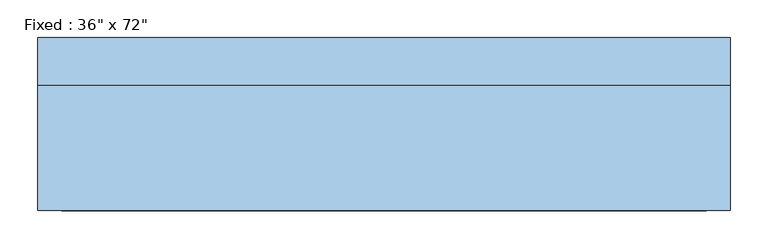
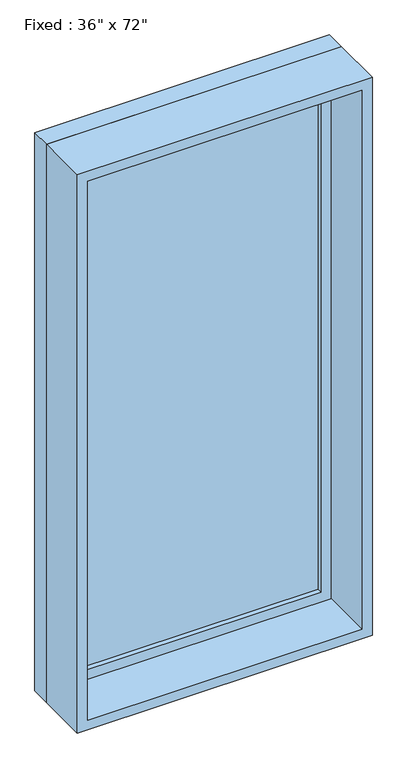
"""IFC4 building model written with IfcOpenShell, lengths in millimetres: window geometry."""

from ifc_helpers import new_model, si_unit, frame, origin, place, context, project, spatial, polyline, outline, extrude, source, transform, mapped, element, save


def window_c796fc87(model_context):
    return source(origin(), model_context, "Body", "SweptSolid", [
        extrude(outline(polyline([(355.6, 66.675), (-431.8, 66.675), (-431.8, 79.375), (355.6, 79.375), (355.6, 66.675)])), frame((0.0, 0.0, 368.3), z_axis=(0.0, 0.0, 1.0), x_axis=(1.0, 0.0, 0.0)), (0.0, 0.0, 1.0), 1701.8),
        extrude(outline(polyline([(2114.55, -476.25), (323.85, -476.25), (323.85, 400.05), (2114.55, 400.05), (2114.55, -476.25)]), holes=[polyline([(2070.1, -431.8), (2070.1, 355.6), (368.3, 355.6), (368.3, -431.8), (2070.1, -431.8)])]), frame((0.0, 50.8, 0.0), z_axis=(0.0, 1.0, 0.0), x_axis=(0.0, 0.0, 1.0)), (0.0, 0.0, 1.0), 44.45),
        extrude(outline(polyline([(2133.6, -495.3), (304.8, -495.3), (304.8, 419.1), (2133.6, 419.1), (2133.6, -495.3)]), holes=[polyline([(2101.85, -463.55), (2101.85, 387.35), (336.55, 387.35), (336.55, -463.55), (2101.85, -463.55)])]), frame((0.0, -114.3, 0.0), z_axis=(0.0, 1.0, 0.0), x_axis=(0.0, 0.0, 1.0)), (0.0, 0.0, 1.0), 165.1),
        extrude(outline(polyline([(2133.6, 419.1), (2133.6, -495.3), (304.8, -495.3), (304.8, 419.1), (2133.6, 419.1)]), holes=[polyline([(2114.55, 400.05), (323.85, 400.05), (323.85, -476.25), (2114.55, -476.25), (2114.55, 400.05)])]), frame((0.0, 50.8, 0.0), z_axis=(0.0, 1.0, 0.0), x_axis=(0.0, 0.0, 1.0)), (0.0, 0.0, 1.0), 63.5),
    ])


if __name__ == "__main__":
    model = new_model("IFC4")
    model_context = context("Model", 3, world=origin())
    ifc_project = project(units=[si_unit("LENGTHUNIT", "METRE", prefix="MILLI")], contexts=[model_context])
    site = spatial("IfcSite", under=ifc_project)
    building = spatial("IfcBuilding", under=site)
    placement = place(None, origin())
    window_shape = window_c796fc87(model_context)
    element("IfcWindow", 1, ObjectType="Fixed : 36\" x 72\"", at=placement, inside=building, context=model_context, shape_type="MappedRepresentation", body=[
        mapped(window_shape, transform((0.0, 0.0, 0.0), x_axis=(1.0, 0.0, 0.0), y_axis=(0.0, 1.0, 0.0), z_axis=(0.0, 0.0, 1.0))),
    ])
    save(model, "model.ifc")

# Revit data of these elements
# Type "Fixed : 36\" x 72\""
#   Type Mark = "9"
#   Construction Type Id = "GSP4R"
#   Assembly Code = "B2020100"
#   Analytic Construction = "1/8 in Pilkington single glazing"
#   Visual Light Transmittance = 0.9
#   Solar Heat Gain Coefficient = 0.78
#   Heat Transfer Coefficient (U) = 0.6496 BTU/(h·ft²·°F)
#   Height = 6' - 0"
#   Default Sill Height = 1' - 0"
#   Width = 3' - 0"
#   Window Inset = 0' - 0 3/4"
#   Define Thermal Properties by = 1
#   Glass Pane Material = Glass
#   Sash Material = Sash
#   Wall Closure = (empty or 0)
# Element 1 (IfcWindow, "Fixed : 36\" x 72\"")
#   Materials on its faces: "Sash", "Glass"
# Materials
#   "Glass": class "Glass", colour RGB 0 128 192, transparency 0.75, Description = "Soda Lime Glass", Cost = 0
#   "Sash": class "Wood", colour RGB 224 178 126, transparency 0
